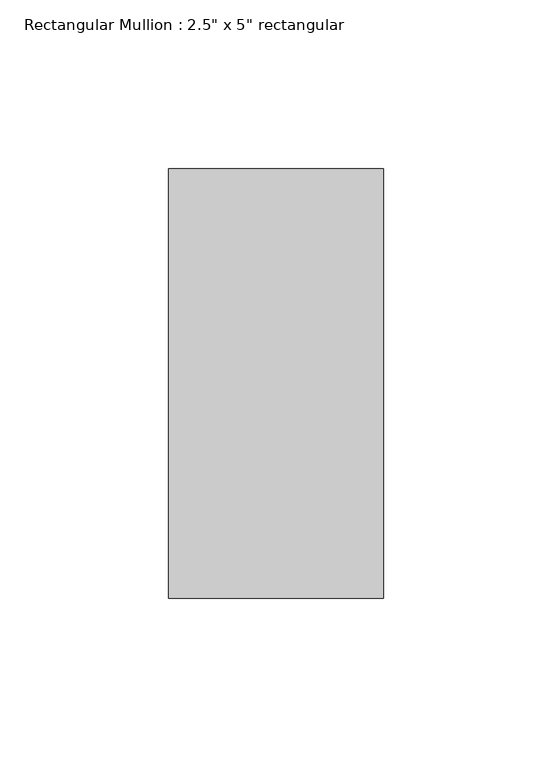
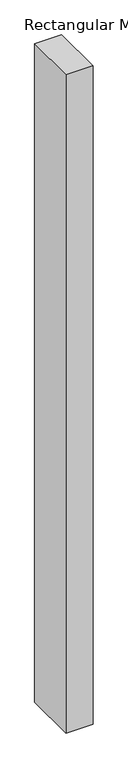
"""IFC4 building model written with IfcOpenShell, lengths in millimetres: member geometry."""

from ifc_helpers import new_model, si_unit, frame, origin, place, context, project, spatial, polyline, outline, extrude, source, transform, mapped, element, save


def member_249e519d(model_context):
    return source(origin(), model_context, "Body", "SweptSolid", [
        extrude(outline(polyline([(0.0, 63.5), (0.0, -63.5), (-63.5, -63.5), (-63.5, 63.5), (0.0, 63.5)])), frame((0.0, 0.0, -1631.95), z_axis=(0.0, 0.0, 1.0), x_axis=(1.0, 0.0, 0.0)), (0.0, 0.0, 1.0), 1631.95),
    ])


if __name__ == "__main__":
    model = new_model("IFC4")
    model_context = context("Model", 3, world=origin())
    ifc_project = project(units=[si_unit("LENGTHUNIT", "METRE", prefix="MILLI")], contexts=[model_context])
    site = spatial("IfcSite", under=ifc_project)
    building = spatial("IfcBuilding", under=site)
    placement = place(None, origin())
    member_shape = member_249e519d(model_context)
    element("IfcMember", 1, ObjectType="Rectangular Mullion : 2.5\" x 5\" rectangular", at=placement, inside=building, context=model_context, shape_type="MappedRepresentation", body=[
        mapped(member_shape, transform((0.0, 0.0, 0.0), x_axis=(1.0, 0.0, 0.0), y_axis=(0.0, 1.0, 0.0), z_axis=(0.0, 0.0, 1.0))),
    ])
    save(model, "model.ifc")

# Revit data of these elements
# Type "Rectangular Mullion : 2.5\" x 5\" rectangular"
#   built-in parameter 1007304 = 0.416667 (stored number, unit not read)
#   built-in parameter 1007301 = 0.104167 (stored number, unit not read)
#   built-in parameter 1007300 = 0.104167 (stored number, unit not read)
# Element 1 (IfcMember, "Rectangular Mullion : 2.5\" x 5\" rectangular")
#   Materials on its faces: "Aluminum"
# Materials
#   "Aluminum": class "Metal", colour RGB 247 247 247, transparency 0, Description = "Aluminum 6061", Cost = 0
